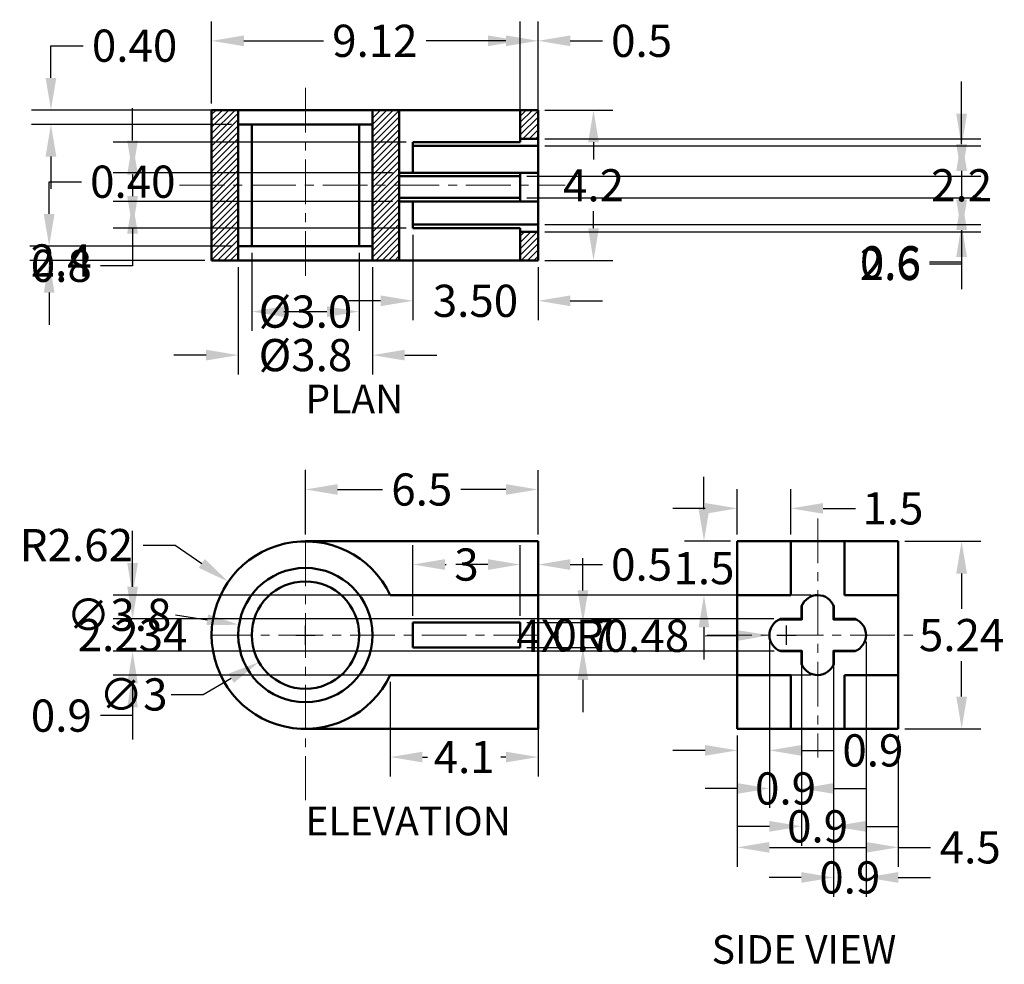
# Model space of a CAD drawing. Units: inches. Extents: x 126.2 to 153.7, y 89.4 to 115.8.
import ezdxf

# ---------------------------------------------------------------- set-up
doc = ezdxf.new("R2010")
doc.units = ezdxf.units.IN
doc.header["$MEASUREMENT"] = 0
doc.linetypes.add('CENTER', pattern=[2, 1.25, -0.25, 0.25, -0.25])
for name, color, linetype, lineweight in [('M-CNTR', 1, 'CENTER', 18), ('M-DIMS', 2, 'Continuous', 25), ('M-HATC', 8, 'Continuous', 18), ('M-OUTL', 7, 'Continuous', 50), ('M-TEXT', 7, 'Continuous', 25)]:
    doc.layers.add(name, color=color, linetype=linetype, lineweight=lineweight)
doc.styles.get("Standard").update_dxf_attribs({"font": 'arial.ttf'})
doc.dimstyles.get("Standard").update_dxf_attribs({"dimscale": 3, "dimtxt": 0.3, "dimasz": 0.3, "dimexe": 0.18, "dimexo": 0.0625, "dimgap": 0.09, "dimtad": 0, "dimtih": 1, "dimtoh": 1, "dimdec": 0, "dimzin": 0, "dimdsep": 46, "dimtxsty": 'Standard', "dimcen": 0.09, "dimclrd": 6, "dimclre": 6, "dimclrt": 3, "dimadec": 0, "dimazin": 0, "dimtfac": 1, "dimtdec": 0, "dimtofl": 0, "dimtmove": 0, "dimatfit": 3, "dimfxl": 1, "dimtolj": 1, "dimtzin": 0, "dimarcsym": 0})
pattern_1 = [(45, (0, 2.72024), (-0.08838835, 0.08838835), [])]

# ---------------------------------------------------------------- blocks, each defined once
blk = doc.blocks.new('*D1')
at = {"layer": 'Defpoints', "color": 0, "transparency": 16777216}
for p in [(140.723, 102.633), (134.223, 101.185), (140.723, 101.185)]:
    blk.add_point(p, dxfattribs=at)
at = {"layer": 'M-DIMS', "color": 0, "lineweight": -2, "transparency": 16777216}
for p, q in [((134.223, 101.373), (134.223, 103.173)), ((140.723, 101.373), (140.723, 103.173)), ((135.123, 102.633), (136.377, 102.633)), ((139.823, 102.633), (138.568, 102.633))]:
    blk.add_line(p, q, dxfattribs=at)
at = {"layer": 'M-DIMS', "color": 0, "transparency": 16777216}
for points in [[(135.123, 102.783), (135.123, 102.483), (134.223, 102.633)], [(139.823, 102.783), (139.823, 102.483), (140.723, 102.633)]]:
    blk.add_solid(points, dxfattribs=at)
at = {"layer": 'M-DIMS', "color": 0, "transparency": 16777216, "insert": (137.473, 102.633), "char_height": 0.9, "attachment_point": 5}
blk.add_mtext('\\A1;6.5', dxfattribs=at)
blk = doc.blocks.new('*D2')
at = {"layer": 'Defpoints', "color": 0, "transparency": 16777216}
for p in [(140.223, 98.915), (141.975, 98.915), (140.223, 98.215)]:
    blk.add_point(p, dxfattribs=at)
at = {"layer": 'M-DIMS', "color": 0, "lineweight": -2, "transparency": 16777216}
for p, q in [((141.975, 99.815), (141.975, 100.715)), ((140.41, 98.915), (142.515, 98.915)), ((140.41, 98.215), (142.515, 98.215)), ((141.975, 97.315), (141.975, 96.415))]:
    blk.add_line(p, q, dxfattribs=at)
at = {"layer": 'M-DIMS', "color": 0, "transparency": 16777216}
for points in [[(141.825, 99.815), (142.125, 99.815), (141.975, 98.915)], [(141.825, 97.315), (142.125, 97.315), (141.975, 98.215)]]:
    blk.add_solid(points, dxfattribs=at)
at = {"layer": 'M-DIMS', "color": 0, "transparency": 16777216, "insert": (141.975, 98.565), "char_height": 0.9, "attachment_point": 5}
blk.add_mtext('\\A1;0.7', dxfattribs=at)
blk = doc.blocks.new('*D3')
at = {"layer": 'Defpoints', "color": 0, "transparency": 16777216}
for p in [(137.223, 100.536), (137.223, 98.915), (140.223, 98.915)]:
    blk.add_point(p, dxfattribs=at)
at = {"layer": 'M-DIMS', "color": 0, "lineweight": -2, "transparency": 16777216}
for p, q in [((137.223, 99.103), (137.223, 101.076)), ((140.223, 99.103), (140.223, 101.076)), ((138.123, 100.536), (138.158, 100.536)), ((139.323, 100.536), (139.287, 100.536))]:
    blk.add_line(p, q, dxfattribs=at)
at = {"layer": 'M-DIMS', "color": 0, "transparency": 16777216}
for points in [[(138.123, 100.686), (138.123, 100.386), (137.223, 100.536)], [(139.323, 100.686), (139.323, 100.386), (140.223, 100.536)]]:
    blk.add_solid(points, dxfattribs=at)
at = {"layer": 'M-DIMS', "color": 0, "transparency": 16777216, "insert": (138.723, 100.536), "char_height": 0.9, "attachment_point": 5}
blk.add_mtext('\\A1;3', dxfattribs=at)
blk = doc.blocks.new('*D4')
at = {"layer": 'Defpoints', "color": 0, "transparency": 16777216}
for p in [(136.593, 97.448), (140.723, 97.448), (140.723, 95.158)]:
    blk.add_point(p, dxfattribs=at)
at = {"layer": 'M-DIMS', "color": 0, "lineweight": -2, "transparency": 16777216}
for p, q in [((136.593, 97.261), (136.593, 94.618)), ((140.723, 97.261), (140.723, 94.618)), ((137.493, 95.158), (137.637, 95.158)), ((139.823, 95.158), (139.678, 95.158))]:
    blk.add_line(p, q, dxfattribs=at)
at = {"layer": 'M-DIMS', "color": 0, "transparency": 16777216}
for points in [[(137.493, 95.308), (137.493, 95.008), (136.593, 95.158)], [(139.823, 95.308), (139.823, 95.008), (140.723, 95.158)]]:
    blk.add_solid(points, dxfattribs=at)
at = {"layer": 'M-DIMS', "color": 0, "transparency": 16777216, "insert": (138.658, 95.158), "char_height": 0.9, "attachment_point": 5}
blk.add_mtext('\\A1;4.1', dxfattribs=at)
blk = doc.blocks.new('*D5')
at = {"layer": 'Defpoints', "color": 0, "transparency": 16777216}
for p in [(140.723, 100.536), (140.223, 99.682), (140.723, 99.682)]:
    blk.add_point(p, dxfattribs=at)
at = {"layer": 'M-DIMS', "color": 0, "lineweight": -2, "transparency": 16777216}
for p, q in [((140.223, 99.87), (140.223, 101.076)), ((140.723, 99.87), (140.723, 101.076)), ((139.323, 100.536), (138.423, 100.536)), ((141.623, 100.536), (142.523, 100.536))]:
    blk.add_line(p, q, dxfattribs=at)
at = {"layer": 'M-DIMS', "color": 0, "transparency": 16777216}
for points in [[(139.323, 100.686), (139.323, 100.386), (140.223, 100.536)], [(141.623, 100.686), (141.623, 100.386), (140.723, 100.536)]]:
    blk.add_solid(points, dxfattribs=at)
at = {"layer": 'M-DIMS', "color": 0, "transparency": 16777216, "insert": (143.615, 100.536), "char_height": 0.9, "attachment_point": 5}
blk.add_mtext('\\A1;0.5', dxfattribs=at)
blk = doc.blocks.new('*D6')
at = {"layer": 'Defpoints', "color": 0, "transparency": 16777216}
for p in [(132.068, 100.056), (134.223, 98.565)]:
    blk.add_point(p, dxfattribs=at)
at = {"layer": 'M-DIMS', "color": 0, "lineweight": -2, "transparency": 16777216}
for p, q in [((129.688, 101.08), (130.588, 101.08)), ((130.588, 101.08), (131.328, 100.568)), ((134.223, 98.295), (134.223, 98.835)), ((133.953, 98.565), (134.493, 98.565))]:
    blk.add_line(p, q, dxfattribs=at)
at = {"layer": 'M-DIMS', "color": 0, "transparency": 16777216}
blk.add_solid([(131.413, 100.691), (131.242, 100.444), (132.068, 100.056)], dxfattribs=at)
at = {"layer": 'M-DIMS', "color": 0, "transparency": 16777216, "insert": (127.823, 101.08), "char_height": 0.9, "attachment_point": 5}
blk.add_mtext('\\A1;R2.62', dxfattribs=at)
blk = doc.blocks.new('*D7')
at = {"layer": 'Defpoints', "color": 0, "transparency": 16777216}
for p in [(132.37, 98.854), (136.075, 98.276)]:
    blk.add_point(p, dxfattribs=at)
at = {"layer": 'M-DIMS', "color": 0, "lineweight": -2, "transparency": 16777216}
for p, q in [((130.592, 99.132), (131.481, 98.993)), ((134.223, 98.295), (134.223, 98.835)), ((133.953, 98.565), (134.493, 98.565))]:
    blk.add_line(p, q, dxfattribs=at)
at = {"layer": 'M-DIMS', "color": 0, "transparency": 16777216}
blk.add_solid([(131.504, 99.142), (131.458, 98.845), (132.37, 98.854)], dxfattribs=at)
at = {"layer": 'M-DIMS', "color": 0, "transparency": 16777216, "insert": (129.012, 99.132), "char_height": 0.9, "attachment_point": 5}
blk.add_mtext('\\A1;∅3.8', dxfattribs=at)
blk = doc.blocks.new('*D8')
at = {"layer": 'Defpoints', "color": 0, "transparency": 16777216}
for p in [(135.519, 99.319), (132.926, 97.811)]:
    blk.add_point(p, dxfattribs=at)
at = {"layer": 'M-DIMS', "color": 0, "lineweight": -2, "transparency": 16777216}
for p, q in [((134.223, 98.295), (134.223, 98.835)), ((133.953, 98.565), (134.493, 98.565)), ((131.369, 96.907), (132.147, 97.359)), ((130.469, 96.907), (131.369, 96.907))]:
    blk.add_line(p, q, dxfattribs=at)
at = {"layer": 'M-DIMS', "color": 0, "transparency": 16777216}
blk.add_solid([(132.072, 97.489), (132.223, 97.23), (132.926, 97.811)], dxfattribs=at)
at = {"layer": 'M-DIMS', "color": 0, "transparency": 16777216, "insert": (129.415, 96.907), "char_height": 0.9, "attachment_point": 5}
blk.add_mtext('\\A1;∅3', dxfattribs=at)
blk = doc.blocks.new('*D9')
at = {"layer": 'Defpoints', "color": 0, "transparency": 16777216}
for p in [(147.786, 102.105), (146.286, 101.185), (147.786, 101.185)]:
    blk.add_point(p, dxfattribs=at)
at = {"layer": 'M-DIMS', "color": 0, "lineweight": -2, "transparency": 16777216}
for p, q in [((146.286, 101.373), (146.286, 102.645)), ((147.786, 101.373), (147.786, 102.645)), ((145.386, 102.105), (144.486, 102.105)), ((148.686, 102.105), (149.586, 102.105))]:
    blk.add_line(p, q, dxfattribs=at)
at = {"layer": 'M-DIMS', "color": 0, "transparency": 16777216}
for points in [[(145.386, 102.255), (145.386, 101.955), (146.286, 102.105)], [(148.686, 102.255), (148.686, 101.955), (147.786, 102.105)]]:
    blk.add_solid(points, dxfattribs=at)
at = {"layer": 'M-DIMS', "color": 0, "transparency": 16777216, "insert": (150.636, 102.105), "char_height": 0.9, "attachment_point": 5}
blk.add_mtext('\\A1;1.5', dxfattribs=at)
blk = doc.blocks.new('*D10')
at = {"layer": 'Defpoints', "color": 0, "transparency": 16777216}
for p in [(146.286, 101.185), (145.357, 99.685), (146.286, 99.685)]:
    blk.add_point(p, dxfattribs=at)
at = {"layer": 'M-DIMS', "color": 0, "lineweight": -2, "transparency": 16777216}
for p, q in [((145.357, 102.085), (145.357, 102.985)), ((146.098, 101.185), (144.817, 101.185)), ((146.098, 99.685), (144.817, 99.685)), ((145.357, 98.785), (145.357, 97.885))]:
    blk.add_line(p, q, dxfattribs=at)
at = {"layer": 'M-DIMS', "color": 0, "transparency": 16777216}
for points in [[(145.207, 102.085), (145.507, 102.085), (145.357, 101.185)], [(145.207, 98.785), (145.507, 98.785), (145.357, 99.685)]]:
    blk.add_solid(points, dxfattribs=at)
at = {"layer": 'M-DIMS', "color": 0, "transparency": 16777216, "insert": (145.357, 100.435), "char_height": 0.9, "attachment_point": 5}
blk.add_mtext('\\A1;1.5', dxfattribs=at)
blk = doc.blocks.new('*D11')
at = {"layer": 'Defpoints', "color": 0, "transparency": 16777216}
for p in [(147.186, 98.562), (146.286, 95.945), (147.186, 95.344)]:
    blk.add_point(p, dxfattribs=at)
at = {"layer": 'M-DIMS', "color": 0, "lineweight": -2, "transparency": 16777216}
for p, q in [((147.186, 98.375), (147.186, 94.804)), ((146.286, 95.758), (146.286, 94.804)), ((145.386, 95.344), (144.486, 95.344)), ((148.086, 95.344), (148.986, 95.344))]:
    blk.add_line(p, q, dxfattribs=at)
at = {"layer": 'M-DIMS', "color": 0, "transparency": 16777216}
for points in [[(145.386, 95.494), (145.386, 95.194), (146.286, 95.344)], [(148.086, 95.494), (148.086, 95.194), (147.186, 95.344)]]:
    blk.add_solid(points, dxfattribs=at)
at = {"layer": 'M-DIMS', "color": 0, "transparency": 16777216, "insert": (150.076, 95.344), "char_height": 0.9, "attachment_point": 5}
blk.add_mtext('\\A1;0.9', dxfattribs=at)
blk = doc.blocks.new('*D12')
at = {"layer": 'Defpoints', "color": 0, "transparency": 16777216}
for p in [(147.186, 98.567), (148.086, 98.115), (148.086, 94.28)]:
    blk.add_point(p, dxfattribs=at)
at = {"layer": 'M-DIMS', "color": 0, "lineweight": -2, "transparency": 16777216}
for p, q in [((147.186, 98.379), (147.186, 93.74)), ((148.086, 97.928), (148.086, 93.74)), ((146.286, 94.28), (145.386, 94.28)), ((148.986, 94.28), (149.886, 94.28))]:
    blk.add_line(p, q, dxfattribs=at)
at = {"layer": 'M-DIMS', "color": 0, "transparency": 16777216}
for points in [[(146.286, 94.43), (146.286, 94.13), (147.186, 94.28)], [(148.986, 94.43), (148.986, 94.13), (148.086, 94.28)]]:
    blk.add_solid(points, dxfattribs=at)
at = {"layer": 'M-DIMS', "color": 0, "transparency": 16777216, "insert": (147.636, 94.28), "char_height": 0.9, "attachment_point": 5}
blk.add_mtext('\\A1;0.9', dxfattribs=at)
blk = doc.blocks.new('*D13')
at = {"layer": 'Defpoints', "color": 0, "transparency": 16777216}
for p in [(148.086, 98.115), (148.976, 98.115), (148.976, 93.222)]:
    blk.add_point(p, dxfattribs=at)
at = {"layer": 'M-DIMS', "color": 0, "lineweight": -2, "transparency": 16777216}
for p, q in [((148.086, 97.928), (148.086, 92.682)), ((148.976, 97.928), (148.976, 92.682)), ((147.186, 93.222), (146.286, 93.222)), ((149.876, 93.222), (150.776, 93.222))]:
    blk.add_line(p, q, dxfattribs=at)
at = {"layer": 'M-DIMS', "color": 0, "transparency": 16777216}
for points in [[(147.186, 93.372), (147.186, 93.072), (148.086, 93.222)], [(149.876, 93.372), (149.876, 93.072), (148.976, 93.222)]]:
    blk.add_solid(points, dxfattribs=at)
at = {"layer": 'M-DIMS', "color": 0, "transparency": 16777216, "insert": (148.531, 93.222), "char_height": 0.9, "attachment_point": 5}
blk.add_mtext('\\A1;0.9', dxfattribs=at)
blk = doc.blocks.new('*D14')
at = {"layer": 'Defpoints', "color": 0, "transparency": 16777216}
for p in [(149.886, 98.567), (148.976, 98.125), (149.886, 91.794)]:
    blk.add_point(p, dxfattribs=at)
at = {"layer": 'M-DIMS', "color": 0, "lineweight": -2, "transparency": 16777216}
for p, q in [((149.886, 98.379), (149.886, 91.254)), ((148.976, 97.938), (148.976, 91.254)), ((148.076, 91.794), (147.176, 91.794)), ((150.786, 91.794), (151.686, 91.794))]:
    blk.add_line(p, q, dxfattribs=at)
at = {"layer": 'M-DIMS', "color": 0, "transparency": 16777216}
for points in [[(148.076, 91.944), (148.076, 91.644), (148.976, 91.794)], [(150.786, 91.944), (150.786, 91.644), (149.886, 91.794)]]:
    blk.add_solid(points, dxfattribs=at)
at = {"layer": 'M-DIMS', "color": 0, "transparency": 16777216, "insert": (149.431, 91.794), "char_height": 0.9, "attachment_point": 5}
blk.add_mtext('\\A1;0.9', dxfattribs=at)
blk = doc.blocks.new('*D15')
at = {"layer": 'Defpoints', "color": 0, "transparency": 16777216}
for p in [(137.223, 109.932), (140.723, 109.032), (140.723, 107.904)]:
    blk.add_point(p, dxfattribs=at)
at = {"layer": 'M-DIMS', "color": 0, "lineweight": -2, "transparency": 16777216}
for p, q in [((137.223, 109.745), (137.223, 107.364)), ((140.723, 108.845), (140.723, 107.364)), ((136.323, 107.904), (135.423, 107.904)), ((141.623, 107.904), (142.523, 107.904))]:
    blk.add_line(p, q, dxfattribs=at)
at = {"layer": 'M-DIMS', "color": 0, "transparency": 16777216}
for points in [[(136.323, 108.054), (136.323, 107.754), (137.223, 107.904)], [(141.623, 108.054), (141.623, 107.754), (140.723, 107.904)]]:
    blk.add_solid(points, dxfattribs=at)
at = {"layer": 'M-DIMS', "color": 0, "transparency": 16777216, "insert": (138.973, 107.904), "char_height": 0.9, "attachment_point": 5}
blk.add_mtext('\\A1;3.50', dxfattribs=at)
blk = doc.blocks.new('*D16')
at = {"layer": 'Defpoints', "color": 0, "transparency": 16777216}
for p in [(132.723, 109.432), (135.723, 109.432), (135.723, 107.603)]:
    blk.add_point(p, dxfattribs=at)
at = {"layer": 'M-DIMS', "color": 0, "lineweight": -2, "transparency": 16777216}
for p, q in [((132.723, 109.245), (132.723, 107.063)), ((135.723, 109.245), (135.723, 107.063)), ((133.623, 107.603), (134.823, 107.603))]:
    blk.add_line(p, q, dxfattribs=at)
at = {"layer": 'M-DIMS', "color": 0, "transparency": 16777216}
for points in [[(133.623, 107.753), (133.623, 107.453), (132.723, 107.603)], [(134.823, 107.753), (134.823, 107.453), (135.723, 107.603)]]:
    blk.add_solid(points, dxfattribs=at)
at = {"layer": 'M-DIMS', "color": 0, "transparency": 16777216, "insert": (134.223, 107.603), "char_height": 0.9, "attachment_point": 5}
blk.add_mtext('\\A1;%%C3.0', dxfattribs=at)
blk = doc.blocks.new('*D17')
at = {"layer": 'Defpoints', "color": 0, "transparency": 16777216}
for p in [(132.348, 109.032), (136.098, 109.032), (136.098, 106.387)]:
    blk.add_point(p, dxfattribs=at)
at = {"layer": 'M-DIMS', "color": 0, "lineweight": -2, "transparency": 16777216}
for p, q in [((132.348, 108.845), (132.348, 105.847)), ((136.098, 108.845), (136.098, 105.847)), ((131.448, 106.387), (130.548, 106.387)), ((136.998, 106.387), (137.898, 106.387))]:
    blk.add_line(p, q, dxfattribs=at)
at = {"layer": 'M-DIMS', "color": 0, "transparency": 16777216}
for points in [[(131.448, 106.537), (131.448, 106.237), (132.348, 106.387)], [(136.998, 106.537), (136.998, 106.237), (136.098, 106.387)]]:
    blk.add_solid(points, dxfattribs=at)
at = {"layer": 'M-DIMS', "color": 0, "transparency": 16777216, "insert": (134.223, 106.387), "char_height": 0.9, "attachment_point": 5}
blk.add_mtext('\\A1;%%C3.8', dxfattribs=at)
blk = doc.blocks.new('*D18')
at = {"layer": 'Defpoints', "color": 0, "transparency": 16777216}
for p in [(127.063, 109.432), (132.348, 109.432), (131.603, 109.032)]:
    blk.add_point(p, dxfattribs=at)
at = {"layer": 'M-DIMS', "color": 0, "lineweight": -2, "transparency": 16777216}
for p, q in [((127.063, 110.332), (127.063, 111.232)), ((127.063, 111.232), (127.963, 111.232)), ((132.16, 109.432), (126.523, 109.432)), ((131.415, 109.032), (126.523, 109.032)), ((127.063, 108.132), (127.063, 107.232))]:
    blk.add_line(p, q, dxfattribs=at)
at = {"layer": 'M-DIMS', "color": 0, "transparency": 16777216}
for points in [[(126.913, 110.332), (127.213, 110.332), (127.063, 109.432)], [(126.913, 108.132), (127.213, 108.132), (127.063, 109.032)]]:
    blk.add_solid(points, dxfattribs=at)
at = {"layer": 'M-DIMS', "color": 0, "transparency": 16777216, "insert": (129.4, 111.232), "char_height": 0.9, "attachment_point": 5}
blk.add_mtext('\\A1;0.40', dxfattribs=at)
blk = doc.blocks.new('*D19')
at = {"layer": 'Defpoints', "color": 0, "transparency": 16777216}
for p in [(127.113, 113.232), (132.348, 113.232), (132.348, 112.832)]:
    blk.add_point(p, dxfattribs=at)
at = {"layer": 'M-DIMS', "color": 0, "lineweight": -2, "transparency": 16777216}
for p, q in [((127.113, 114.132), (127.113, 115.032)), ((127.113, 115.032), (128.013, 115.032)), ((132.16, 113.232), (126.573, 113.232)), ((132.16, 112.832), (126.573, 112.832)), ((127.113, 111.932), (127.113, 111.032))]:
    blk.add_line(p, q, dxfattribs=at)
at = {"layer": 'M-DIMS', "color": 0, "transparency": 16777216}
for points in [[(126.963, 114.132), (127.263, 114.132), (127.113, 113.232)], [(126.963, 111.932), (127.263, 111.932), (127.113, 112.832)]]:
    blk.add_solid(points, dxfattribs=at)
at = {"layer": 'M-DIMS', "color": 0, "transparency": 16777216, "insert": (129.45, 115.032), "char_height": 0.9, "attachment_point": 5}
blk.add_mtext('\\A1;0.40', dxfattribs=at)
blk = doc.blocks.new('*D20')
at = {"layer": 'Defpoints', "color": 0, "transparency": 16777216}
for p in [(140.723, 113.232), (140.723, 109.032), (142.271, 109.032)]:
    blk.add_point(p, dxfattribs=at)
at = {"layer": 'M-DIMS', "color": 0, "lineweight": -2, "transparency": 16777216}
for p, q in [((140.91, 113.232), (142.811, 113.232)), ((142.271, 112.332), (142.271, 111.854)), ((142.271, 109.932), (142.271, 110.41)), ((140.91, 109.032), (142.811, 109.032))]:
    blk.add_line(p, q, dxfattribs=at)
at = {"layer": 'M-DIMS', "color": 0, "transparency": 16777216}
for points in [[(142.121, 112.332), (142.421, 112.332), (142.271, 113.232)], [(142.121, 109.932), (142.421, 109.932), (142.271, 109.032)]]:
    blk.add_solid(points, dxfattribs=at)
at = {"layer": 'M-DIMS', "color": 0, "transparency": 16777216, "insert": (142.271, 111.132), "char_height": 0.9, "attachment_point": 5}
blk.add_mtext('\\A1;4.2', dxfattribs=at)
blk = doc.blocks.new('*D21')
at = {"layer": 'Defpoints', "color": 0, "transparency": 16777216}
for p in [(140.723, 112.432), (140.723, 109.832), (152.555, 109.832)]:
    blk.add_point(p, dxfattribs=at)
at = {"layer": 'M-DIMS', "color": 6, "lineweight": -2, "transparency": 16777216}
for p, q in [((140.91, 112.432), (153.095, 112.432)), ((152.555, 111.532), (152.555, 110.732)), ((140.91, 109.832), (153.095, 109.832)), ((152.555, 109.832), (152.555, 108.932)), ((152.555, 108.932), (151.655, 108.932))]:
    blk.add_line(p, q, dxfattribs=at)
at = {"layer": 'M-DIMS', "color": 6, "transparency": 16777216}
for points in [[(152.405, 111.532), (152.705, 111.532), (152.555, 112.432)], [(152.405, 110.732), (152.705, 110.732), (152.555, 109.832)]]:
    blk.add_solid(points, dxfattribs=at)
at = {"layer": 'M-DIMS', "color": 3, "transparency": 16777216, "insert": (150.558, 108.932), "char_height": 0.9, "attachment_point": 5}
blk.add_mtext('\\A1;2.6', dxfattribs=at)
blk = doc.blocks.new('*D22')
at = {"layer": 'Defpoints', "color": 0, "transparency": 16777216}
for p in [(140.722537, 112.232339), (140.722537, 110.032339), (152.554728, 110.032339)]:
    blk.add_point(p, dxfattribs=at)
at = {"layer": 'M-DIMS', "color": 6, "lineweight": -2, "transparency": 16777216}
for p, q in [((152.554728, 113.132339), (152.554728, 114.032339)), ((140.910037, 112.232339), (153.094728, 112.232339)), ((140.910037, 110.032339), (153.094728, 110.032339)), ((152.554728, 109.132339), (152.554728, 108.232339))]:
    blk.add_line(p, q, dxfattribs=at)
at = {"layer": 'M-DIMS', "color": 6, "transparency": 16777216}
for points in [[(152.404728, 113.132339), (152.704728, 113.132339), (152.554728, 112.232339)], [(152.404728, 109.132339), (152.704728, 109.132339), (152.554728, 110.032339)]]:
    blk.add_solid(points, dxfattribs=at)
at = {"layer": 'M-DIMS', "color": 3, "transparency": 16777216, "insert": (152.554728, 111.132339), "char_height": 0.9, "attachment_point": 5}
blk.add_mtext('\\A1;2.2', dxfattribs=at)
blk = doc.blocks.new('*D23')
at = {"layer": 'Defpoints', "color": 0, "transparency": 16777216}
for p in [(136.843, 111.482), (129.393, 110.682), (136.843, 110.682)]:
    blk.add_point(p, dxfattribs=at)
at = {"layer": 'M-DIMS', "color": 6, "lineweight": -2, "transparency": 16777216}
for p, q in [((129.393, 112.382), (129.393, 113.282)), ((136.655, 111.482), (128.853, 111.482)), ((136.655, 110.682), (128.853, 110.682)), ((129.393, 109.782), (129.393, 108.882)), ((129.393, 108.882), (128.493, 108.882))]:
    blk.add_line(p, q, dxfattribs=at)
at = {"layer": 'M-DIMS', "color": 6, "transparency": 16777216}
for points in [[(129.243, 112.382), (129.543, 112.382), (129.393, 111.482)], [(129.243, 109.782), (129.543, 109.782), (129.393, 110.682)]]:
    blk.add_solid(points, dxfattribs=at)
at = {"layer": 'M-DIMS', "color": 3, "transparency": 16777216, "insert": (127.403, 108.882), "char_height": 0.9, "attachment_point": 5}
blk.add_mtext('\\A1;0.8', dxfattribs=at)
blk = doc.blocks.new('*D24')
at = {"layer": 'Defpoints', "color": 0, "transparency": 16777216}
for p in [(137.223, 112.332), (129.393, 109.932), (137.223, 109.932)]:
    blk.add_point(p, dxfattribs=at)
at = {"layer": 'M-DIMS', "color": 6, "lineweight": -2, "transparency": 16777216}
for p, q in [((137.035, 112.332), (128.853, 112.332)), ((129.393, 111.432), (129.393, 110.832)), ((137.035, 109.932), (128.853, 109.932)), ((129.393, 109.932), (129.393, 109.032)), ((129.393, 109.032), (128.493, 109.032))]:
    blk.add_line(p, q, dxfattribs=at)
at = {"layer": 'M-DIMS', "color": 6, "transparency": 16777216}
for points in [[(129.243, 111.432), (129.543, 111.432), (129.393, 112.332)], [(129.243, 110.832), (129.543, 110.832), (129.393, 109.932)]]:
    blk.add_solid(points, dxfattribs=at)
at = {"layer": 'M-DIMS', "color": 3, "transparency": 16777216, "insert": (127.398, 109.032), "char_height": 0.9, "attachment_point": 5}
blk.add_mtext('\\A1;2.4', dxfattribs=at)
blk = doc.blocks.new('*D25')
at = {"layer": 'Defpoints', "color": 0, "transparency": 16777216}
for p in [(140.223, 111.382), (140.223, 110.782), (152.555, 110.782)]:
    blk.add_point(p, dxfattribs=at)
at = {"layer": 'M-DIMS', "color": 6, "lineweight": -2, "transparency": 16777216}
for p, q in [((152.555, 112.282), (152.555, 113.182)), ((140.41, 111.382), (153.095, 111.382)), ((140.41, 110.782), (153.095, 110.782)), ((152.555, 109.882), (152.555, 108.982)), ((152.555, 108.982), (151.655, 108.982))]:
    blk.add_line(p, q, dxfattribs=at)
at = {"layer": 'M-DIMS', "color": 6, "transparency": 16777216}
for points in [[(152.405, 112.282), (152.705, 112.282), (152.555, 111.382)], [(152.405, 109.882), (152.705, 109.882), (152.555, 110.782)]]:
    blk.add_solid(points, dxfattribs=at)
at = {"layer": 'M-DIMS', "color": 3, "transparency": 16777216, "insert": (150.566, 108.982), "char_height": 0.9, "attachment_point": 5}
blk.add_mtext('\\A1;0.6', dxfattribs=at)
blk = doc.blocks.new('*D26')
at = {"layer": 'Defpoints', "color": 0, "transparency": 16777216}
for p in [(140.723, 115.168), (140.223, 112.432), (140.723, 112.432)]:
    blk.add_point(p, dxfattribs=at)
at = {"layer": 'M-DIMS', "color": 6, "lineweight": -2, "transparency": 16777216}
for p, q in [((140.223, 112.62), (140.223, 115.708)), ((140.723, 112.62), (140.723, 115.708)), ((139.323, 115.168), (138.423, 115.168)), ((141.623, 115.168), (142.523, 115.168))]:
    blk.add_line(p, q, dxfattribs=at)
at = {"layer": 'M-DIMS', "color": 6, "transparency": 16777216}
for points in [[(139.323, 115.318), (139.323, 115.018), (140.223, 115.168)], [(141.623, 115.318), (141.623, 115.018), (140.723, 115.168)]]:
    blk.add_solid(points, dxfattribs=at)
at = {"layer": 'M-DIMS', "color": 3, "transparency": 16777216, "insert": (143.615, 115.168), "char_height": 0.9, "attachment_point": 5}
blk.add_mtext('\\A1;0.5', dxfattribs=at)
blk = doc.blocks.new('*D27')
at = {"layer": 'Defpoints', "color": 0, "transparency": 16777216}
for p in [(148.538, 99.682), (129.393, 97.448), (148.538, 97.448)]:
    blk.add_point(p, dxfattribs=at)
at = {"layer": 'M-DIMS', "color": 6, "lineweight": -2, "transparency": 16777216}
for p, q in [((129.393, 100.582), (129.393, 101.482)), ((148.351, 99.682), (128.853, 99.682)), ((148.351, 97.448), (128.853, 97.448)), ((129.393, 96.548), (129.393, 95.648))]:
    blk.add_line(p, q, dxfattribs=at)
at = {"layer": 'M-DIMS', "color": 6, "transparency": 16777216}
for points in [[(129.243, 100.582), (129.543, 100.582), (129.393, 99.682)], [(129.243, 96.548), (129.543, 96.548), (129.393, 97.448)]]:
    blk.add_solid(points, dxfattribs=at)
at = {"layer": 'M-DIMS', "color": 3, "transparency": 16777216, "insert": (129.393, 98.565), "char_height": 0.9, "attachment_point": 5}
blk.add_mtext('\\A1;2.234', dxfattribs=at)
blk = doc.blocks.new('*D28')
at = {"layer": 'Defpoints', "color": 0, "transparency": 16777216}
for p in [(147.493, 99.015), (129.393, 98.115), (147.502, 98.115)]:
    blk.add_point(p, dxfattribs=at)
at = {"layer": 'M-DIMS', "color": 6, "lineweight": -2, "transparency": 16777216}
for p, q in [((129.393, 99.915), (129.393, 100.815)), ((147.306, 99.015), (128.853, 99.015)), ((147.314, 98.115), (128.853, 98.115)), ((129.393, 97.215), (129.393, 96.315)), ((129.393, 96.315), (128.493, 96.315))]:
    blk.add_line(p, q, dxfattribs=at)
at = {"layer": 'M-DIMS', "color": 6, "transparency": 16777216}
for points in [[(129.243, 99.915), (129.543, 99.915), (129.393, 99.015)], [(129.243, 97.215), (129.543, 97.215), (129.393, 98.115)]]:
    blk.add_solid(points, dxfattribs=at)
at = {"layer": 'M-DIMS', "color": 3, "transparency": 16777216, "insert": (127.403, 96.315), "char_height": 0.9, "attachment_point": 5}
blk.add_mtext('\\A1;0.9', dxfattribs=at)
blk = doc.blocks.new('*D29')
at = {"layer": 'Defpoints', "color": 0, "transparency": 16777216}
for p in [(150.786, 101.185), (150.786, 95.945), (152.555, 95.945)]:
    blk.add_point(p, dxfattribs=at)
at = {"layer": 'M-DIMS', "color": 6, "lineweight": -2, "transparency": 16777216}
for p, q in [((150.973, 101.185), (153.095, 101.185)), ((152.555, 100.285), (152.555, 99.295)), ((152.555, 96.845), (152.555, 97.836)), ((150.973, 95.945), (153.095, 95.945))]:
    blk.add_line(p, q, dxfattribs=at)
at = {"layer": 'M-DIMS', "color": 6, "transparency": 16777216}
for points in [[(152.405, 100.285), (152.705, 100.285), (152.555, 101.185)], [(152.405, 96.845), (152.705, 96.845), (152.555, 95.945)]]:
    blk.add_solid(points, dxfattribs=at)
at = {"layer": 'M-DIMS', "color": 3, "transparency": 16777216, "insert": (152.555, 98.565), "char_height": 0.9, "attachment_point": 5}
blk.add_mtext('\\A1;5.24', dxfattribs=at)
blk = doc.blocks.new('*D30')
at = {"layer": 'Defpoints', "color": 0, "transparency": 16777216}
for p in [(146.286, 95.945), (150.786, 95.945), (150.786, 92.635)]:
    blk.add_point(p, dxfattribs=at)
at = {"layer": 'M-DIMS', "color": 6, "lineweight": -2, "transparency": 16777216}
for p, q in [((146.286, 95.758), (146.286, 92.095)), ((150.786, 95.758), (150.786, 92.095)), ((147.186, 92.635), (149.886, 92.635)), ((150.786, 92.635), (151.686, 92.635))]:
    blk.add_line(p, q, dxfattribs=at)
at = {"layer": 'M-DIMS', "color": 6, "transparency": 16777216}
for points in [[(147.186, 92.785), (147.186, 92.485), (146.286, 92.635)], [(149.886, 92.785), (149.886, 92.485), (150.786, 92.635)]]:
    blk.add_solid(points, dxfattribs=at)
at = {"layer": 'M-DIMS', "color": 3, "transparency": 16777216, "insert": (152.796, 92.635), "char_height": 0.9, "attachment_point": 5}
blk.add_mtext('\\A1;4.5', dxfattribs=at)
blk = doc.blocks.new('*D31')
at = {"layer": 'Defpoints', "color": 0, "transparency": 16777216}
for p in [(140.723, 115.168), (131.603, 113.232), (140.723, 113.232)]:
    blk.add_point(p, dxfattribs=at)
at = {"layer": 'M-DIMS', "color": 6, "lineweight": -2, "transparency": 16777216}
for p, q in [((131.603, 113.42), (131.603, 115.708)), ((140.723, 113.42), (140.723, 115.708)), ((132.503, 115.168), (134.728, 115.168)), ((139.823, 115.168), (137.597, 115.168))]:
    blk.add_line(p, q, dxfattribs=at)
at = {"layer": 'M-DIMS', "color": 6, "transparency": 16777216}
for points in [[(132.503, 115.318), (132.503, 115.018), (131.603, 115.168)], [(139.823, 115.318), (139.823, 115.018), (140.723, 115.168)]]:
    blk.add_solid(points, dxfattribs=at)
at = {"layer": 'M-DIMS', "color": 3, "transparency": 16777216, "insert": (136.163, 115.168), "char_height": 0.9, "attachment_point": 5}
blk.add_mtext('\\A1;9.12', dxfattribs=at)
blk = doc.blocks.new('*D32')
at = {"layer": 'Defpoints', "color": 0, "transparency": 16777216}
for p in [(147.186, 98.562), (147.666, 98.567)]:
    blk.add_point(p, dxfattribs=at)
at = {"layer": 'M-DIMS', "color": 6, "lineweight": -2, "transparency": 16777216}
for p, q in [((147.666, 98.297), (147.666, 98.837)), ((145.386, 98.545), (146.286, 98.553)), ((147.396, 98.567), (147.936, 98.567))]:
    blk.add_line(p, q, dxfattribs=at)
at = {"layer": 'M-DIMS', "color": 6, "transparency": 16777216}
blk.add_solid([(146.284, 98.703), (146.287, 98.403), (147.186, 98.562)], dxfattribs=at)
at = {"layer": 'M-DIMS', "color": 3, "transparency": 16777216, "insert": (142.53, 98.545), "char_height": 0.9, "attachment_point": 5}
blk.add_mtext('\\A1;4X R0.48', dxfattribs=at)

msp = doc.modelspace()

# ---------------------------------------------------------------- hatches: boundary and pattern name
at = {"layer": 'M-HATC'}
h = msp.add_hatch(dxfattribs=at)
h.set_pattern_fill('ANSI31', color=256)
h.set_pattern_definition(pattern_1)
h.paths.add_polyline_path([(131.6025, 109.0323), (132.3475, 109.0323), (132.3475, 113.2323), (131.6025, 113.2323)])
h.paths.add_polyline_path([(136.0975, 109.0323), (136.8425, 109.0323), (136.8425, 113.2323), (136.0975, 113.2323), (136.0975, 112.8323)])
h = msp.add_hatch(dxfattribs=at)
h.set_pattern_fill('ANSI31', color=256)
h.set_pattern_definition(pattern_1)
h.paths.add_polyline_path([(140.2225, 109.0323), (140.7225, 109.0323), (140.7225, 109.8323), (140.2225, 109.8323)])
h.paths.add_polyline_path([(140.2225, 112.4323), (140.7225, 112.4323), (140.7225, 113.2323), (140.2225, 113.2323)])

# ---------------------------------------------------------------- linework, layer by layer
at = {"layer": 'M-CNTR'}
for p, q in [((134.2225, 113.8526), (134.2225, 108.4121)), ((130.7077, 111.1323), (141.48, 111.1323)), ((134.2225, 103.1797), (134.2225, 93.9505)), ((148.5355, 101.82), (148.5355, 95.1456)), ((140.7225, 98.5651), (131.6025, 98.5651)), ((145.4422, 98.5651), (151.2397, 98.5651))]:
    msp.add_line(p, q, dxfattribs=at)
at = {"layer": 'M-OUTL'}
for p, q in [((131.6025, 113.2323), (131.6025, 109.0323)), ((132.3475, 113.2323), (131.6025, 113.2323)), ((132.3475, 113.2323), (132.3475, 109.0323)), ((136.0975, 113.2323), (136.0975, 109.0323)), ((136.0975, 113.2323), (136.8425, 113.2323)), ((136.8425, 113.2323), (136.8425, 109.0323)), ((136.8425, 113.2323), (140.7225, 113.2323)), ((140.2225, 112.3323), (140.2225, 113.2323)), ((140.7225, 109.0323), (140.7225, 113.2323)), ((132.7225, 112.8323), (132.7225, 109.4323)), ((132.7225, 112.8323), (135.7225, 112.8323)), ((135.7225, 112.8323), (135.7225, 109.4323)), ((137.2225, 112.3323), (137.2225, 111.4823)), ((137.2225, 112.3323), (140.2225, 112.3323)), ((137.2225, 112.2323), (140.7225, 112.2323)), ((140.2225, 112.4323), (140.7225, 112.4323)), ((136.8425, 111.4823), (140.7225, 111.4823)), ((140.2225, 110.6823), (140.2225, 111.4823)), ((136.8425, 111.3823), (140.2225, 111.3823)), ((136.8425, 110.7823), (140.2225, 110.7823)), ((136.8425, 110.6823), (140.7225, 110.6823)), ((137.2225, 110.6823), (137.2225, 109.9323)), ((137.2225, 110.0323), (140.7225, 110.0323)), ((137.2225, 109.9323), (140.2225, 109.9323)), ((140.2225, 109.9323), (140.2225, 109.0323)), ((140.2225, 109.8323), (140.7225, 109.8323)), ((132.7225, 109.4323), (135.7225, 109.4323)), ((132.3475, 109.0323), (131.6025, 109.0323)), ((136.0975, 109.0323), (136.8425, 109.0323)), ((136.8425, 109.0323), (140.7225, 109.0323)), ((140.7225, 101.1851), (134.2225, 101.1851)), ((140.7225, 101.1851), (140.7225, 95.9451)), ((146.2855, 101.1851), (146.2855, 95.9451)), ((146.2855, 101.1851), (150.7855, 101.1851)), ((147.7855, 101.1851), (147.7855, 99.6851)), ((149.2855, 101.1851), (149.2855, 99.6851)), ((150.7855, 101.1851), (150.7855, 95.9451)), ((136.5925, 99.682), (140.7225, 99.682)), ((146.2855, 99.6851), (147.7855, 99.6851)), ((149.2855, 99.6851), (150.7855, 99.6851)), ((140.2225, 98.9151), (137.2225, 98.9151)), ((137.2225, 98.9151), (137.2225, 98.2151)), ((140.2225, 98.9151), (140.2225, 98.2151)), ((140.2225, 98.2151), (137.2225, 98.2151)), ((136.5925, 97.4482), (140.7225, 97.4482)), ((146.2855, 97.4451), (147.7855, 97.4451)), ((147.7855, 97.4451), (147.7855, 95.9451)), ((149.2855, 97.4451), (150.7855, 97.4451)), ((149.2855, 97.4451), (149.2855, 95.9451)), ((140.7225, 95.9451), (134.2225, 95.9451)), ((146.2855, 95.9451), (150.7855, 95.9451))]:
    msp.add_line(p, q, dxfattribs=at)
for points in [[(132.3475, 113.2323), (136.0975, 113.2323), (136.0975, 112.8323), (132.3475, 112.8323)], [(132.3475, 109.0323), (136.0975, 109.0323), (136.0975, 109.4323), (132.3475, 109.4323)]]:
    msp.add_lwpolyline(points, close=True, dxfattribs=at)
for points in [[(147.4694, 99.0051), (148.0955, 99.0051), (148.0955, 99.3981)], [(147.4934, 99.0151), (148.0855, 99.0151), (148.0855, 99.3741)], [(148.9755, 99.391), (148.9755, 99.0051), (149.6017, 99.0051)], [(148.9855, 99.3657), (148.9855, 99.0151), (149.5776, 99.0151)], [(147.4766, 98.1251), (148.0955, 98.1251), (148.0955, 97.732)], [(147.5018, 98.1151), (148.0855, 98.1151), (148.0855, 97.7561)], [(148.9755, 97.7392), (148.9755, 98.1251), (149.5945, 98.1251)], [(148.9855, 97.7645), (148.9855, 98.1151), (149.5692, 98.1151)]]:
    msp.add_lwpolyline(points, dxfattribs=at)
for radius in [1.875, 1.5]:
    msp.add_circle((134.2225, 98.5651), radius, dxfattribs=at)
for centre, radius, start, end in [((134.2225, 98.5651), 2.62, 25.2332, 334.7668), ((148.5339, 99.2015), 0.4805, 19.98292, 158.94562), ((147.666, 98.5667), 0.4805, 111.05438, 250.01708), ((149.405, 98.5667), 0.4805, 289.98292, 68.94562), ((148.5339, 97.9287), 0.4805, 201.05438, 340.01708)]:
    msp.add_arc(centre, radius, start, end, dxfattribs=at)

# ---------------------------------------------------------------- texts
at = {"layer": 'M-TEXT', "char_height": 0.8, "attachment_point": 1}
for s, width, insert in [('PLAN', 4.63855, (134.2225, 105.5624)), ('ELEVATION', 4.63855, (134.2225, 93.7693)), ('SIDE VIEW', 5.790643, (145.5728, 90.1817))]:
    msp.add_mtext_dynamic_manual_height_columns(s, width=width, gutter_width=1, heights=[0], dxfattribs=dict(at, insert=insert))

# ---------------------------------------------------------------- dimensions: what is measured, and where the dimension line sits
at = {"layer": 'M-DIMS'}
for base, p1, p2, override, picture, middle in [((127.1126, 113.2323), (132.3475, 112.8323), (132.3475, 113.2323), {"dimdec": 2, "dimclrd": 0, "dimclre": 0, "dimclrt": 0}, '*D19', (129.4499, 115.0323)), ((152.5547, 110.0323), (140.7225, 112.2323), (140.7225, 110.0323), {"dimdec": 1, "dimlfac": 1, "dimrnd": 0, "dimzin": 0, "dimdsep": 46, "dimlunit": 2}, '*D22', (152.5547, 111.1323)), ((129.3927, 110.6823), (136.8425, 111.4823), (136.8425, 110.6823), {"dimdec": 1, "dimlfac": 1, "dimrnd": 0, "dimzin": 0, "dimdsep": 46, "dimlunit": 2}, '*D23', (127.4025, 108.8823)), ((152.5547, 110.7823), (140.2225, 111.3823), (140.2225, 110.7823), {"dimdec": 1, "dimlfac": 1, "dimrnd": 0, "dimzin": 0, "dimdsep": 46, "dimlunit": 2}, '*D25', (150.5658, 108.9823)), ((142.2705, 109.0323), (140.7225, 113.2323), (140.7225, 109.0323), {"dimdec": 1, "dimclrd": 0, "dimclre": 0, "dimclrt": 0}, '*D20', (142.2705, 111.1323)), ((129.3927, 109.9323), (137.2225, 112.3323), (137.2225, 109.9323), {"dimdec": 1, "dimlfac": 1, "dimrnd": 0, "dimzin": 0, "dimdsep": 46, "dimlunit": 2}, '*D24', (127.3976, 109.0323)), ((152.5547, 109.8323), (140.7225, 112.4323), (140.7225, 109.8323), {"dimdec": 1, "dimlfac": 1, "dimrnd": 0, "dimzin": 0, "dimdsep": 46, "dimlunit": 2}, '*D21', (150.5581, 108.9323)), ((145.3567, 99.6851), (146.2855, 101.1851), (146.2855, 99.6851), {"dimdec": 1, "dimclrd": 0, "dimclre": 0, "dimclrt": 0}, '*D10', (145.3567, 100.4351)), ((129.3927, 97.4482), (148.5384, 99.682), (148.5384, 97.4482), {"dimdec": 3, "dimlfac": 1, "dimrnd": 0, "dimzin": 0, "dimdsep": 46, "dimlunit": 2}, '*D27', (129.3927, 98.5651)), ((152.5547, 95.9451), (150.7855, 101.1851), (150.7855, 95.9451), {"dimdec": 2, "dimlfac": 1, "dimrnd": 0, "dimzin": 0, "dimdsep": 46, "dimlunit": 2}, '*D29', (152.5547, 98.5651)), ((129.3927, 98.1151), (147.4934, 99.0151), (147.5018, 98.1151), {"dimdec": 1, "dimlfac": 1, "dimrnd": 0, "dimzin": 0, "dimdsep": 46, "dimlunit": 2}, '*D28', (127.4025, 96.3151))]:
    dim = msp.add_linear_dim(base=base, p1=p1, p2=p2, angle=90, dimstyle='Standard', override=override, dxfattribs=at)
    dim.commit()
    dim.dimension.update_dxf_attribs({"geometry": picture, "text_midpoint": middle})
for base, p1, p2, override, picture, middle in [((140.7225, 115.1676), (131.6025, 113.2323), (140.7225, 113.2323), {"dimdec": 2, "dimlfac": 1, "dimrnd": 0, "dimzin": 0, "dimdsep": 46, "dimlunit": 2}, '*D31', (136.1625, 115.1676)), ((140.7225, 115.1676), (140.2225, 112.4323), (140.7225, 112.4323), {"dimdec": 1, "dimlfac": 1, "dimrnd": 0, "dimzin": 0, "dimdsep": 46, "dimlunit": 2}, '*D26', (143.6152, 115.1676)), ((140.7225, 102.6329), (134.2225, 101.1851), (140.7225, 101.1851), {"dimdec": 1, "dimclrd": 0, "dimclre": 0, "dimclrt": 0}, '*D1', (137.4725, 102.6329)), ((147.7855, 102.1051), (146.2855, 101.1851), (147.7855, 101.1851), {"dimdec": 1, "dimclrd": 0, "dimclre": 0, "dimclrt": 0}, '*D9', (150.6358, 102.1051)), ((140.7225, 100.5358), (140.2225, 99.682), (140.7225, 99.682), {"dimdec": 1, "dimclrd": 0, "dimclre": 0, "dimclrt": 0}, '*D5', (143.6152, 100.5358)), ((147.1855, 95.3435), (146.2855, 95.9451), (147.1855, 98.5622), {"dimdec": 1, "dimclrd": 0, "dimclre": 0, "dimclrt": 0}, '*D11', (150.0757, 95.3435)), ((150.7855, 92.6355), (146.2855, 95.9451), (150.7855, 95.9451), {"dimdec": 1, "dimlfac": 1, "dimrnd": 0, "dimzin": 0, "dimdsep": 46, "dimlunit": 2}, '*D30', (152.7963, 92.6355))]:
    dim = msp.add_linear_dim(base=base, p1=p1, p2=p2, dimstyle='Standard', override=override, dxfattribs=at)
    dim.commit()
    dim.dimension.update_dxf_attribs({"geometry": picture, "text_midpoint": middle})
for base, p1, p2, override, picture, middle in [((127.0628, 109.4323), (131.6025, 109.0323), (132.3475, 109.4323), {"dimdec": 2, "dimclrd": 0, "dimclre": 0, "dimclrt": 0}, '*D18', (129.4002, 111.2323)), ((141.9748, 98.9151), (140.2225, 98.2151), (140.2225, 98.9151), {"dimdec": 1, "dimclrd": 0, "dimclre": 0, "dimclrt": 0}, '*D2', (141.9748, 98.5651))]:
    dim = msp.add_linear_dim(base=base, p1=p1, p2=p2, angle=90, dimstyle='Standard', override=override, dxfattribs=at)
    dim.commit()
    dim.dimension.update_dxf_attribs({"geometry": picture, "text_midpoint": middle, "dimtype": 160})
for base, p1, p2, override, picture, middle in [((140.7225, 107.9038), (137.2225, 109.9323), (140.7225, 109.0323), {"dimdec": 2, "dimclrd": 0, "dimclre": 0, "dimclrt": 0}, '*D15', (138.9725, 107.9038)), ((137.2225, 100.5358), (140.2225, 98.9151), (137.2225, 98.9151), {"dimclrd": 0, "dimclre": 0, "dimclrt": 0}, '*D3', (138.7225, 100.5358)), ((148.0855, 94.2797), (147.1855, 98.5667), (148.0855, 98.1151), {"dimdec": 1, "dimclrd": 0, "dimclre": 0, "dimclrt": 0}, '*D12', (147.6355, 94.2797)), ((149.8855, 91.7935), (148.9755, 98.1251), (149.8855, 98.5667), {"dimdec": 1, "dimclrd": 0, "dimclre": 0, "dimclrt": 0}, '*D14', (149.4305, 91.7935)), ((148.9755, 93.222), (148.0855, 98.1151), (148.9755, 98.1151), {"dimdec": 1, "dimclrd": 0, "dimclre": 0, "dimclrt": 0}, '*D13', (148.5305, 93.222)), ((140.7225, 95.158), (136.5925, 97.4482), (140.7225, 97.4482), {"dimdec": 1, "dimclrd": 0, "dimclre": 0, "dimclrt": 0}, '*D4', (138.6575, 95.158))]:
    dim = msp.add_linear_dim(base=base, p1=p1, p2=p2, dimstyle='Standard', override=override, dxfattribs=at)
    dim.commit()
    dim.dimension.update_dxf_attribs({"geometry": picture, "text_midpoint": middle, "dimtype": 160})
for base, p1, p2, picture, middle in [((135.7225, 107.603), (132.7225, 109.4323), (135.7225, 109.4323), '*D16', (134.2225, 107.603)), ((136.0975374016, 106.3874408249), (132.3475374016, 109.032339445), (136.0975374016, 109.032339445), '*D17', (134.2225374016, 106.3874408249))]:
    dim = msp.add_linear_dim(base=base, p1=p1, p2=p2, text='%%C<>', dimstyle='Standard', override={"dimdec": 1, "dimclrd": 0, "dimclre": 0, "dimclrt": 0}, dxfattribs=at)
    dim.commit()
    dim.dimension.update_dxf_attribs({"geometry": picture, "text_midpoint": middle, "dimtype": 160})
dim = msp.add_radius_dim(center=(134.2225, 98.5651), mpoint=(132.0679, 100.0557), dimstyle='Standard', override={"dimdec": 2, "dimclrd": 0, "dimclre": 0, "dimclrt": 0}, dxfattribs=at)
dim.commit()
dim.dimension.update_dxf_attribs({"geometry": '*D6', "text_midpoint": (127.8227, 101.0798)})
dim = msp.add_radius_dim(center=(147.666, 98.5667), mpoint=(147.1855, 98.562), text='4X <>', dimstyle='Standard', override={"dimdec": 2, "dimlfac": 1, "dimrnd": 0, "dimzin": 0, "dimdsep": 46, "dimlunit": 2}, dxfattribs=at)
dim.commit()
dim.dimension.update_dxf_attribs({"geometry": '*D32', "text_midpoint": (142.5301, 98.5445)})
for p1, p2, override, picture, middle in [((136.0750698, 98.2756949), (132.370005, 98.8544819), {"dimdec": 1, "dimclrd": 0, "dimclre": 0, "dimclrt": 0}, '*D7', (129.0117853, 99.1322997)), ((135.5195, 99.3187), (132.9256, 97.8114), {"dimclrd": 0, "dimclre": 0, "dimclrt": 0}, '*D8', (129.4147, 96.9071))]:
    dim = msp.add_diameter_dim_2p(p1=p1, p2=p2, dimstyle='Standard', override=override, dxfattribs=at)
    dim.commit()
    dim.dimension.update_dxf_attribs({"geometry": picture, "text_midpoint": middle})

doc.saveas('drawing.dxf')
